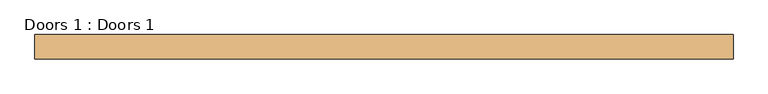
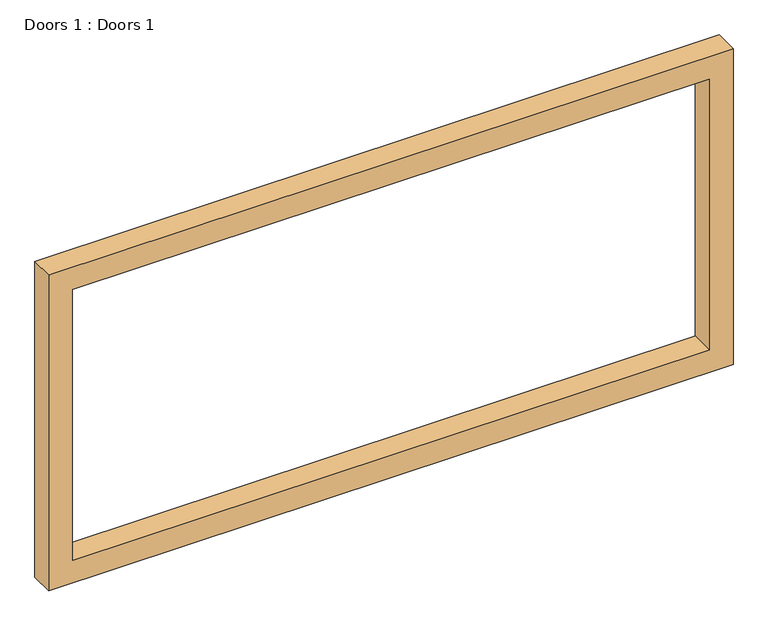
"""IFC4 building model written with IfcOpenShell, lengths in millimetres: door geometry, Doors 1 : Doors 1."""

from ifc_helpers import new_model, si_unit, frame, origin, place, context, project, spatial, polyline, outline, extrude, source, transform, mapped, element, save


def doors_1_doors_1_af7bef9e(model_context):
    return source(origin(), model_context, "Body", "SweptSolid", [
        extrude(outline(polyline([(13106.4, -7590.8388186), (13106.4, -16328.4388186), (8839.2, -16328.4388186), (8839.2, -7590.8388186), (13106.4, -7590.8388186)]), holes=[polyline([(12801.6, -7895.6388186), (9144.0, -7895.6388186), (9144.0, -16023.6388186), (12801.6, -16023.6388186), (12801.6, -7895.6388186)])]), frame((0.0, -261.8548049, 0.0), z_axis=(0.0, 1.0, 0.0), x_axis=(0.0, 0.0, 1.0)), (0.0, 0.0, 1.0), 304.8),
    ])


if __name__ == "__main__":
    model = new_model("IFC4")
    model_context = context("Model", 3, world=origin())
    ifc_project = project(units=[si_unit("LENGTHUNIT", "METRE", prefix="MILLI")], contexts=[model_context])
    site = spatial("IfcSite", under=ifc_project)
    building = spatial("IfcBuilding", under=site)
    placement = place(None, origin())
    doors_1_doors_1_shape = doors_1_doors_1_af7bef9e(model_context)
    element("IfcDoor", 1, ObjectType="Doors 1 : Doors 1", at=placement, inside=building, context=model_context, shape_type="MappedRepresentation", body=[
        mapped(doors_1_doors_1_shape, transform((0.0, 0.0, 0.0), x_axis=(1.0, 0.0, 0.0), y_axis=(0.0, 1.0, 0.0), z_axis=(0.0, 0.0, 1.0))),
    ])
    save(model, "model.ifc")

# Revit data of these elements
# Type "Doors 1 : Doors 1"
#   Type Mark = "8"
# Element 1 (IfcDoor, "Doors 1 : Doors 1")
#   Materials on its faces: "Default New Material(1)"
# Materials
#   "Default New Material(1)": class "Generic", colour RGB 157 111 8, transparency 0, Cost = 0
